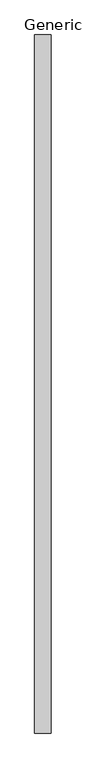
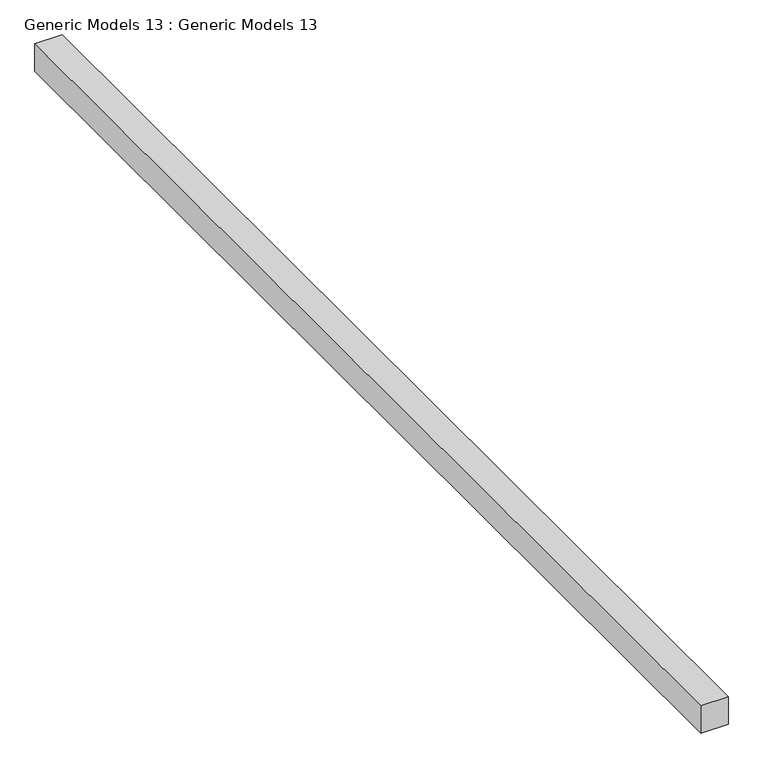
"""IFC4 building model written with IfcOpenShell, lengths in millimetres: proxy geometry, Generic Models 13 : Generic Models 13."""

from ifc_helpers import new_model, si_unit, frame, origin, place, context, project, spatial, polyline, outline, extrude, source, transform, mapped, element, save


def generic_models_13_generic_models_13_7be0e28e(model_context):
    return source(origin(), model_context, "Body", "SweptSolid", [
        extrude(outline(polyline([(-15581.438074, -5966.8213044), (-15581.438074, 6898.2537088), (-15276.638074, 6898.2537088), (-15276.638074, -5966.8213044), (-15581.438074, -5966.8213044)])), frame((0.0, 0.0, 32519.7385091), z_axis=(0.0, 0.0, 1.0), x_axis=(1.0, 0.0, 0.0)), (0.0, 0.0, 1.0), 320.898547),
    ])


if __name__ == "__main__":
    model = new_model("IFC4")
    model_context = context("Model", 3, world=origin())
    ifc_project = project(units=[si_unit("LENGTHUNIT", "METRE", prefix="MILLI")], contexts=[model_context])
    site = spatial("IfcSite", under=ifc_project)
    building = spatial("IfcBuilding", under=site)
    placement = place(None, origin())
    generic_models_13_generic_models_13_shape = generic_models_13_generic_models_13_7be0e28e(model_context)
    element("IfcBuildingElementProxy", 1, Name="Generic Models 13 : Generic Models 13", ObjectType="Generic Models 13 : Generic Models 13", at=placement, inside=building, context=model_context, shape_type="MappedRepresentation", body=[
        mapped(generic_models_13_generic_models_13_shape, transform((0.0, 0.0, 0.0), x_axis=(1.0, 0.0, 0.0), y_axis=(0.0, 1.0, 0.0), z_axis=(0.0, 0.0, 1.0))),
    ])
    save(model, "model.ifc")
